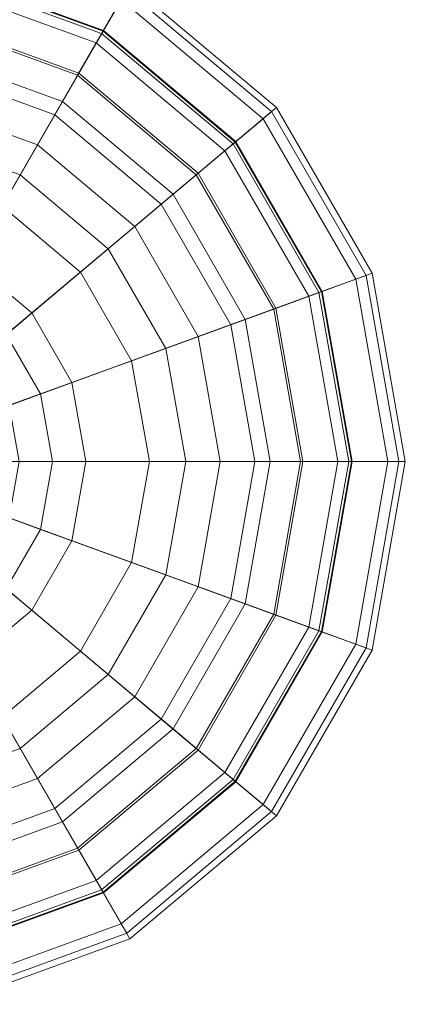
# Model space of a CAD drawing. Units: inches. Extents: x 375 to 1122, y 27 to 1069.
# Tile 121 of 155: x 719.669 to 720.617, y 889.781 to 892.201. Entities that reach past the tile are written whole.
import ezdxf

# ---------------------------------------------------------------- set-up
doc = ezdxf.new("R2010")
doc.units = ezdxf.units.IN
doc.layers.add('Furniture', color=30, linetype='Continuous', lineweight=18)

# ---------------------------------------------------------------- blocks, each defined once
blk = doc.blocks.new('A$C403C54AD')
for points in [[(1.180252, 0.891746, -0.031825), (1.180252, 0.857884, -0.028747), (1.180252, 0.857884, -0.028747), (1.16867, 0.889704, -0.031825)], [(1.180252, 0.88848, -0.028594), (1.180252, 0.891746, -0.031825), (1.16867, 0.889704, -0.031825), (1.169787, 0.886635, -0.028594)], [(1.180252, 0.88844, 0.131159), (1.180252, 0.891347, 0.117935), (1.168807, 0.889329, 0.117935), (1.169801, 0.886597, 0.131159)], [(1.180252, 0.891347, 0.117935), (1.180252, 0.890672, 0.089693), (1.169038, 0.888695, 0.089693), (1.168807, 0.889329, 0.117935)], [(1.191834, 0.889704, -0.031825), (1.180252, 0.857884, -0.028747), (1.180252, 0.857884, -0.028747), (1.180252, 0.891746, -0.031825)], [(1.190717, 0.886635, -0.028594), (1.191834, 0.889704, -0.031825), (1.180252, 0.891746, -0.031825), (1.180252, 0.88848, -0.028594)], [(1.190703, 0.886597, 0.131159), (1.191697, 0.889329, 0.117935), (1.180252, 0.891347, 0.117935), (1.180252, 0.88844, 0.131159)], [(1.191697, 0.889329, 0.117935), (1.191466, 0.888695, 0.089693), (1.180252, 0.890672, 0.089693), (1.180252, 0.891347, 0.117935)], [(1.180252, 0.890672, 0.089693), (1.180252, 0.885308, 0.071684), (1.170873, 0.883654, 0.071684), (1.169038, 0.888695, 0.089693)], [(1.191466, 0.888695, 0.089693), (1.189632, 0.883654, 0.071684), (1.180252, 0.885308, 0.071684), (1.180252, 0.890672, 0.089693)], [(1.169787, 0.886635, -0.028594), (1.16867, 0.889704, -0.031825), (1.158486, 0.883824, -0.031825), (1.160585, 0.881322, -0.028594)], [(1.16867, 0.889704, -0.031825), (1.180252, 0.857884, -0.028747), (1.180252, 0.857884, -0.028747), (1.158486, 0.883824, -0.031825)], [(1.202018, 0.883824, -0.031825), (1.180252, 0.857884, -0.028747), (1.180252, 0.857884, -0.028747), (1.191834, 0.889704, -0.031825)], [(1.199919, 0.881322, -0.028594), (1.202018, 0.883824, -0.031825), (1.191834, 0.889704, -0.031825), (1.190717, 0.886635, -0.028594)], [(1.169801, 0.886597, 0.131159), (1.168807, 0.889329, 0.117935), (1.158742, 0.883518, 0.117935), (1.160611, 0.881291, 0.131159)], [(1.168807, 0.889329, 0.117935), (1.169038, 0.888695, 0.089693), (1.159176, 0.883001, 0.089693), (1.158742, 0.883518, 0.117935)], [(1.199893, 0.881291, 0.131159), (1.201762, 0.883518, 0.117935), (1.191697, 0.889329, 0.117935), (1.190703, 0.886597, 0.131159)], [(1.201762, 0.883518, 0.117935), (1.201328, 0.883001, 0.089693), (1.191466, 0.888695, 0.089693), (1.191697, 0.889329, 0.117935)], [(1.169038, 0.888695, 0.089693), (1.170873, 0.883654, 0.071684), (1.162624, 0.878892, 0.071684), (1.159176, 0.883001, 0.089693)], [(1.180252, 0.872098, -0.02532), (1.180252, 0.88848, -0.028594), (1.169787, 0.886635, -0.028594), (1.17539, 0.871241, -0.02532)], [(1.180252, 0.883444, 0.140564), (1.180252, 0.88844, 0.131159), (1.169801, 0.886597, 0.131159), (1.17151, 0.881902, 0.140564)], [(1.185114, 0.871241, -0.02532), (1.190717, 0.886635, -0.028594), (1.180252, 0.88848, -0.028594), (1.180252, 0.872098, -0.02532)], [(1.188994, 0.881902, 0.140564), (1.190703, 0.886597, 0.131159), (1.180252, 0.88844, 0.131159), (1.180252, 0.883444, 0.140564)], [(1.201328, 0.883001, 0.089693), (1.19788, 0.878892, 0.071684), (1.189632, 0.883654, 0.071684), (1.191466, 0.888695, 0.089693)], [(1.180252, 0.888263, 0.117718), (1.180252, 0.885453, 0.130354), (1.170823, 0.88379, 0.130354), (1.169862, 0.886431, 0.117718)], [(1.180252, 0.887605, 0.090178), (1.180252, 0.888263, 0.117718), (1.169862, 0.886431, 0.117718), (1.170087, 0.885812, 0.090178)], [(1.190642, 0.886431, 0.117718), (1.189681, 0.88379, 0.130354), (1.180252, 0.885453, 0.130354), (1.180252, 0.888263, 0.117718)], [(1.190417, 0.885812, 0.090178), (1.190642, 0.886431, 0.117718), (1.180252, 0.888263, 0.117718), (1.180252, 0.887605, 0.090178)], [(1.180252, 0.882497, 0.073031), (1.180252, 0.887605, 0.090178), (1.170087, 0.885812, 0.090178), (1.171834, 0.881013, 0.073031)], [(1.18867, 0.881013, 0.073031), (1.190417, 0.885812, 0.090178), (1.180252, 0.887605, 0.090178), (1.180252, 0.882497, 0.073031)], [(1.17539, 0.871241, -0.02532), (1.169787, 0.886635, -0.028594), (1.160585, 0.881322, -0.028594), (1.171115, 0.868773, -0.02532)], [(1.17151, 0.881902, 0.140564), (1.169801, 0.886597, 0.131159), (1.160611, 0.881291, 0.131159), (1.163823, 0.877464, 0.140564)], [(1.189389, 0.868773, -0.02532), (1.199919, 0.881322, -0.028594), (1.190717, 0.886635, -0.028594), (1.185114, 0.871241, -0.02532)], [(1.196681, 0.877464, 0.140564), (1.199893, 0.881291, 0.131159), (1.190703, 0.886597, 0.131159), (1.188994, 0.881902, 0.140564)], [(1.169862, 0.886431, 0.117718), (1.170823, 0.88379, 0.130354), (1.162531, 0.879003, 0.130354), (1.160725, 0.881156, 0.117718)], [(1.170087, 0.885812, 0.090178), (1.169862, 0.886431, 0.117718), (1.160725, 0.881156, 0.117718), (1.161148, 0.880651, 0.090178)], [(1.199779, 0.881156, 0.117718), (1.197973, 0.879003, 0.130354), (1.189681, 0.88379, 0.130354), (1.190642, 0.886431, 0.117718)], [(1.199356, 0.880651, 0.090178), (1.199779, 0.881156, 0.117718), (1.190642, 0.886431, 0.117718), (1.190417, 0.885812, 0.090178)], [(1.171834, 0.881013, 0.073031), (1.170087, 0.885812, 0.090178), (1.161148, 0.880651, 0.090178), (1.164431, 0.876739, 0.073031)], [(1.180252, 0.885453, 0.130354), (1.180252, 0.880365, 0.140564), (1.172563, 0.879009, 0.140564), (1.170823, 0.88379, 0.130354)], [(1.180252, 0.885308, 0.071684), (1.180252, 0.878242, 0.061451), (1.173289, 0.877014, 0.061451), (1.170873, 0.883654, 0.071684)], [(1.189681, 0.88379, 0.130354), (1.187941, 0.879009, 0.140564), (1.180252, 0.880365, 0.140564), (1.180252, 0.885453, 0.130354)], [(1.189632, 0.883654, 0.071684), (1.187215, 0.877014, 0.061451), (1.180252, 0.878242, 0.061451), (1.180252, 0.885308, 0.071684)], [(1.196073, 0.876739, 0.073031), (1.199356, 0.880651, 0.090178), (1.190417, 0.885812, 0.090178), (1.18867, 0.881013, 0.073031)], [(1.160585, 0.881322, -0.028594), (1.158486, 0.883824, -0.031825), (1.150927, 0.874815, -0.031825), (1.153755, 0.873182, -0.028594)], [(1.158486, 0.883824, -0.031825), (1.180252, 0.857884, -0.028747), (1.180252, 0.857884, -0.028747), (1.150927, 0.874815, -0.031825)], [(1.160611, 0.881291, 0.131159), (1.158742, 0.883518, 0.117935), (1.151272, 0.874616, 0.117935), (1.15379, 0.873162, 0.131159)], [(1.158742, 0.883518, 0.117935), (1.159176, 0.883001, 0.089693), (1.151856, 0.874278, 0.089693), (1.151272, 0.874616, 0.117935)], [(1.170823, 0.88379, 0.130354), (1.172563, 0.879009, 0.140564), (1.165801, 0.875106, 0.140564), (1.162531, 0.879003, 0.130354)], [(1.170873, 0.883654, 0.071684), (1.173289, 0.877014, 0.061451), (1.167166, 0.873479, 0.061451), (1.162624, 0.878892, 0.071684)], [(1.180252, 0.880365, 0.140564), (1.180252, 0.883444, 0.140564), (1.17151, 0.881902, 0.140564), (1.172563, 0.879009, 0.140564)], [(1.209578, 0.874815, -0.031825), (1.180252, 0.857884, -0.028747), (1.180252, 0.857884, -0.028747), (1.202018, 0.883824, -0.031825)], [(1.187941, 0.879009, 0.140564), (1.188994, 0.881902, 0.140564), (1.180252, 0.883444, 0.140564), (1.180252, 0.880365, 0.140564)], [(1.19788, 0.878892, 0.071684), (1.193338, 0.873479, 0.061451), (1.187215, 0.877014, 0.061451), (1.189632, 0.883654, 0.071684)], [(1.197973, 0.879003, 0.130354), (1.194703, 0.875106, 0.140564), (1.187941, 0.879009, 0.140564), (1.189681, 0.88379, 0.130354)], [(1.206714, 0.873162, 0.131159), (1.209232, 0.874616, 0.117935), (1.201762, 0.883518, 0.117935), (1.199893, 0.881291, 0.131159)], [(1.206749, 0.873182, -0.028594), (1.209578, 0.874815, -0.031825), (1.202018, 0.883824, -0.031825), (1.199919, 0.881322, -0.028594)], [(1.209232, 0.874616, 0.117935), (1.208648, 0.874278, 0.089693), (1.201328, 0.883001, 0.089693), (1.201762, 0.883518, 0.117935)], [(1.159176, 0.883001, 0.089693), (1.162624, 0.878892, 0.071684), (1.156502, 0.871596, 0.071684), (1.151856, 0.874278, 0.089693)], [(1.208648, 0.874278, 0.089693), (1.204002, 0.871596, 0.071684), (1.19788, 0.878892, 0.071684), (1.201328, 0.883001, 0.089693)], [(1.180252, 0.876011, 0.063639), (1.180252, 0.882497, 0.073031), (1.171834, 0.881013, 0.073031), (1.174052, 0.874918, 0.063639)], [(1.186452, 0.874918, 0.063639), (1.18867, 0.881013, 0.073031), (1.180252, 0.882497, 0.073031), (1.180252, 0.876011, 0.063639)], [(1.172563, 0.879009, 0.140564), (1.17151, 0.881902, 0.140564), (1.163823, 0.877464, 0.140564), (1.165801, 0.875106, 0.140564)], [(1.194703, 0.875106, 0.140564), (1.196681, 0.877464, 0.140564), (1.188994, 0.881902, 0.140564), (1.187941, 0.879009, 0.140564)], [(1.171115, 0.868773, -0.02532), (1.160585, 0.881322, -0.028594), (1.153755, 0.873182, -0.028594), (1.167942, 0.864991, -0.02532)], [(1.163823, 0.877464, 0.140564), (1.160611, 0.881291, 0.131159), (1.15379, 0.873162, 0.131159), (1.158117, 0.870664, 0.140564)], [(1.160725, 0.881156, 0.117718), (1.162531, 0.879003, 0.130354), (1.156376, 0.871669, 0.130354), (1.153943, 0.873073, 0.117718)], [(1.161148, 0.880651, 0.090178), (1.160725, 0.881156, 0.117718), (1.153943, 0.873073, 0.117718), (1.154513, 0.872744, 0.090178)], [(1.174052, 0.874918, 0.063639), (1.171834, 0.881013, 0.073031), (1.164431, 0.876739, 0.073031), (1.1686, 0.87177, 0.063639)], [(1.191904, 0.87177, 0.063639), (1.196073, 0.876739, 0.073031), (1.18867, 0.881013, 0.073031), (1.186452, 0.874918, 0.063639)], [(1.192562, 0.864991, -0.02532), (1.206749, 0.873182, -0.028594), (1.199919, 0.881322, -0.028594), (1.189389, 0.868773, -0.02532)], [(1.202387, 0.870664, 0.140564), (1.206714, 0.873162, 0.131159), (1.199893, 0.881291, 0.131159), (1.196681, 0.877464, 0.140564)], [(1.206561, 0.873073, 0.117718), (1.204128, 0.871669, 0.130354), (1.197973, 0.879003, 0.130354), (1.199779, 0.881156, 0.117718)], [(1.205991, 0.872744, 0.090178), (1.206561, 0.873073, 0.117718), (1.199779, 0.881156, 0.117718), (1.199356, 0.880651, 0.090178)], [(1.164431, 0.876739, 0.073031), (1.161148, 0.880651, 0.090178), (1.154513, 0.872744, 0.090178), (1.158936, 0.87019, 0.073031)], [(1.201568, 0.87019, 0.073031), (1.205991, 0.872744, 0.090178), (1.199356, 0.880651, 0.090178), (1.196073, 0.876739, 0.073031)], [(1.162531, 0.879003, 0.130354), (1.165801, 0.875106, 0.140564), (1.160783, 0.869125, 0.140564), (1.156376, 0.871669, 0.130354)], [(1.162624, 0.878892, 0.071684), (1.167166, 0.873479, 0.061451), (1.162622, 0.868063, 0.061451), (1.156502, 0.871596, 0.071684)], [(1.204002, 0.871596, 0.071684), (1.197882, 0.868063, 0.061451), (1.193338, 0.873479, 0.061451), (1.19788, 0.878892, 0.071684)], [(1.204128, 0.871669, 0.130354), (1.199721, 0.869125, 0.140564), (1.194703, 0.875106, 0.140564), (1.197973, 0.879003, 0.130354)], [(1.180252, 0.878242, 0.061451), (1.180252, 0.868003, 0.054084), (1.176791, 0.867392, 0.054084), (1.173289, 0.877014, 0.061451)], [(1.187215, 0.877014, 0.061451), (1.183713, 0.867392, 0.054084), (1.180252, 0.868003, 0.054084), (1.180252, 0.878242, 0.061451)], [(1.165801, 0.875106, 0.140564), (1.163823, 0.877464, 0.140564), (1.158117, 0.870664, 0.140564), (1.160783, 0.869125, 0.140564)], [(1.199721, 0.869125, 0.140564), (1.202387, 0.870664, 0.140564), (1.196681, 0.877464, 0.140564), (1.194703, 0.875106, 0.140564)], [(1.173289, 0.877014, 0.061451), (1.176791, 0.867392, 0.054084), (1.173748, 0.865635, 0.054084), (1.167166, 0.873479, 0.061451)], [(1.193338, 0.873479, 0.061451), (1.186756, 0.865635, 0.054084), (1.183713, 0.867392, 0.054084), (1.187215, 0.877014, 0.061451)], [(1.1686, 0.87177, 0.063639), (1.164431, 0.876739, 0.073031), (1.158936, 0.87019, 0.073031), (1.164553, 0.866948, 0.063639)], [(1.195951, 0.866948, 0.063639), (1.201568, 0.87019, 0.073031), (1.196073, 0.876739, 0.073031), (1.191904, 0.87177, 0.063639)], [(1.180252, 0.866788, 0.057003), (1.180252, 0.876011, 0.063639), (1.174052, 0.874918, 0.063639), (1.177207, 0.866251, 0.057003)], [(1.183297, 0.866251, 0.057003), (1.186452, 0.874918, 0.063639), (1.180252, 0.876011, 0.063639), (1.180252, 0.866788, 0.057003)], [(1.153755, 0.873182, -0.028594), (1.150927, 0.874815, -0.031825), (1.146904, 0.863764, -0.031825), (1.15012, 0.863197, -0.028594)], [(1.150927, 0.874815, -0.031825), (1.180252, 0.857884, -0.028747), (1.180252, 0.857884, -0.028747), (1.146904, 0.863764, -0.031825)], [(1.15379, 0.873162, 0.131159), (1.151272, 0.874616, 0.117935), (1.147297, 0.863695, 0.117935), (1.15016, 0.86319, 0.131159)], [(1.177207, 0.866251, 0.057003), (1.174052, 0.874918, 0.063639), (1.1686, 0.87177, 0.063639), (1.174529, 0.864705, 0.057003)], [(1.2136, 0.863764, -0.031825), (1.180252, 0.857884, -0.028747), (1.180252, 0.857884, -0.028747), (1.209578, 0.874815, -0.031825)], [(1.185975, 0.864705, 0.057003), (1.191904, 0.87177, 0.063639), (1.186452, 0.874918, 0.063639), (1.183297, 0.866251, 0.057003)], [(1.210344, 0.86319, 0.131159), (1.213207, 0.863695, 0.117935), (1.209232, 0.874616, 0.117935), (1.206714, 0.873162, 0.131159)], [(1.210384, 0.863197, -0.028594), (1.2136, 0.863764, -0.031825), (1.209578, 0.874815, -0.031825), (1.206749, 0.873182, -0.028594)], [(1.213207, 0.863695, 0.117935), (1.212542, 0.863578, 0.089693), (1.208648, 0.874278, 0.089693), (1.209232, 0.874616, 0.117935)], [(1.151856, 0.874278, 0.089693), (1.156502, 0.871596, 0.071684), (1.153245, 0.862646, 0.071684), (1.147962, 0.863578, 0.089693)], [(1.212542, 0.863578, 0.089693), (1.207259, 0.862646, 0.071684), (1.204002, 0.871596, 0.071684), (1.208648, 0.874278, 0.089693)], [(1.167942, 0.864991, -0.02532), (1.153755, 0.873182, -0.028594), (1.15012, 0.863197, -0.028594), (1.166254, 0.860352, -0.02532)], [(1.158117, 0.870664, 0.140564), (1.15379, 0.873162, 0.131159), (1.15016, 0.86319, 0.131159), (1.155081, 0.862322, 0.140564)], [(1.167166, 0.873479, 0.061451), (1.173748, 0.865635, 0.054084), (1.171489, 0.862943, 0.054084), (1.162622, 0.868063, 0.061451)], [(1.197882, 0.868063, 0.061451), (1.189015, 0.862943, 0.054084), (1.186756, 0.865635, 0.054084), (1.193338, 0.873479, 0.061451)], [(1.19425, 0.860352, -0.02532), (1.210384, 0.863197, -0.028594), (1.206749, 0.873182, -0.028594), (1.192562, 0.864991, -0.02532)], [(1.205423, 0.862322, 0.140564), (1.210344, 0.86319, 0.131159), (1.206714, 0.873162, 0.131159), (1.202387, 0.870664, 0.140564)], [(1.153943, 0.873073, 0.117718), (1.156376, 0.871669, 0.130354), (1.153102, 0.862671, 0.130354), (1.150335, 0.863159, 0.117718)], [(1.154513, 0.872744, 0.090178), (1.153943, 0.873073, 0.117718), (1.150335, 0.863159, 0.117718), (1.150983, 0.863045, 0.090178)], [(1.158936, 0.87019, 0.073031), (1.154513, 0.872744, 0.090178), (1.150983, 0.863045, 0.090178), (1.156013, 0.862158, 0.073031)], [(1.204491, 0.862158, 0.073031), (1.209521, 0.863045, 0.090178), (1.205991, 0.872744, 0.090178), (1.201568, 0.87019, 0.073031)], [(1.210169, 0.863159, 0.117718), (1.207402, 0.862671, 0.130354), (1.204128, 0.871669, 0.130354), (1.206561, 0.873073, 0.117718)], [(1.209521, 0.863045, 0.090178), (1.210169, 0.863159, 0.117718), (1.206561, 0.873073, 0.117718), (1.205991, 0.872744, 0.090178)], [(1.180252, 0.87005, -0.022455), (1.180252, 0.872098, -0.02532), (1.17539, 0.871241, -0.02532), (1.176091, 0.869317, -0.022455)], [(1.184413, 0.869317, -0.022455), (1.185114, 0.871241, -0.02532), (1.180252, 0.872098, -0.02532), (1.180252, 0.87005, -0.022455)], [(1.156376, 0.871669, 0.130354), (1.160783, 0.869125, 0.140564), (1.158112, 0.861788, 0.140564), (1.153102, 0.862671, 0.130354)], [(1.156502, 0.871596, 0.071684), (1.162622, 0.868063, 0.061451), (1.160204, 0.861419, 0.061451), (1.153245, 0.862646, 0.071684)], [(1.174529, 0.864705, 0.057003), (1.1686, 0.87177, 0.063639), (1.164553, 0.866948, 0.063639), (1.172541, 0.862336, 0.057003)], [(1.187963, 0.862336, 0.057003), (1.195951, 0.866948, 0.063639), (1.191904, 0.87177, 0.063639), (1.185975, 0.864705, 0.057003)], [(1.207259, 0.862646, 0.071684), (1.2003, 0.861419, 0.061451), (1.197882, 0.868063, 0.061451), (1.204002, 0.871596, 0.071684)], [(1.207402, 0.862671, 0.130354), (1.202392, 0.861788, 0.140564), (1.199721, 0.869125, 0.140564), (1.204128, 0.871669, 0.130354)], [(1.176091, 0.869317, -0.022455), (1.17539, 0.871241, -0.02532), (1.171115, 0.868773, -0.02532), (1.172432, 0.867204, -0.022455)], [(1.188073, 0.867204, -0.022455), (1.189389, 0.868773, -0.02532), (1.185114, 0.871241, -0.02532), (1.184413, 0.869317, -0.022455)], [(1.160783, 0.869125, 0.140564), (1.158117, 0.870664, 0.140564), (1.155081, 0.862322, 0.140564), (1.158112, 0.861788, 0.140564)], [(1.164553, 0.866948, 0.063639), (1.158936, 0.87019, 0.073031), (1.156013, 0.862158, 0.073031), (1.1624, 0.861032, 0.063639)], [(1.198104, 0.861032, 0.063639), (1.204491, 0.862158, 0.073031), (1.201568, 0.87019, 0.073031), (1.195951, 0.866948, 0.063639)], [(1.202392, 0.861788, 0.140564), (1.205423, 0.862322, 0.140564), (1.202387, 0.870664, 0.140564), (1.199721, 0.869125, 0.140564)], [(1.180252, 0.865955, -0.020408), (1.180252, 0.87005, -0.022455), (1.176091, 0.869317, -0.022455), (1.177492, 0.865468, -0.020408)], [(1.183012, 0.865468, -0.020408), (1.184413, 0.869317, -0.022455), (1.180252, 0.87005, -0.022455), (1.180252, 0.865955, -0.020408)], [(1.177492, 0.865468, -0.020408), (1.176091, 0.869317, -0.022455), (1.172432, 0.867204, -0.022455), (1.175064, 0.864067, -0.020408)], [(1.18544, 0.864067, -0.020408), (1.188073, 0.867204, -0.022455), (1.184413, 0.869317, -0.022455), (1.183012, 0.865468, -0.020408)], [(1.172432, 0.867204, -0.022455), (1.171115, 0.868773, -0.02532), (1.167942, 0.864991, -0.02532), (1.169716, 0.863967, -0.022455)], [(1.190789, 0.863967, -0.022455), (1.192562, 0.864991, -0.02532), (1.189389, 0.868773, -0.02532), (1.188073, 0.867204, -0.022455)], [(1.162622, 0.868063, 0.061451), (1.171489, 0.862943, 0.054084), (1.170287, 0.859641, 0.054084), (1.160204, 0.861419, 0.061451)], [(1.2003, 0.861419, 0.061451), (1.190217, 0.859641, 0.054084), (1.189015, 0.862943, 0.054084), (1.197882, 0.868063, 0.061451)]]:
    blk.add_3dface(points)

msp = doc.modelspace()

# ---------------------------------------------------------------- block references
at = {"layer": 'Furniture', "xscale": 39.9918517141215, "yscale": 39.9918517141215, "zscale": 39.9918517141215, "rotation": 270}
msp.add_blockref('A$C403C54AD', (684.9549, 938.3156, 0.024), dxfattribs=at)

doc.saveas('drawing.dxf')
